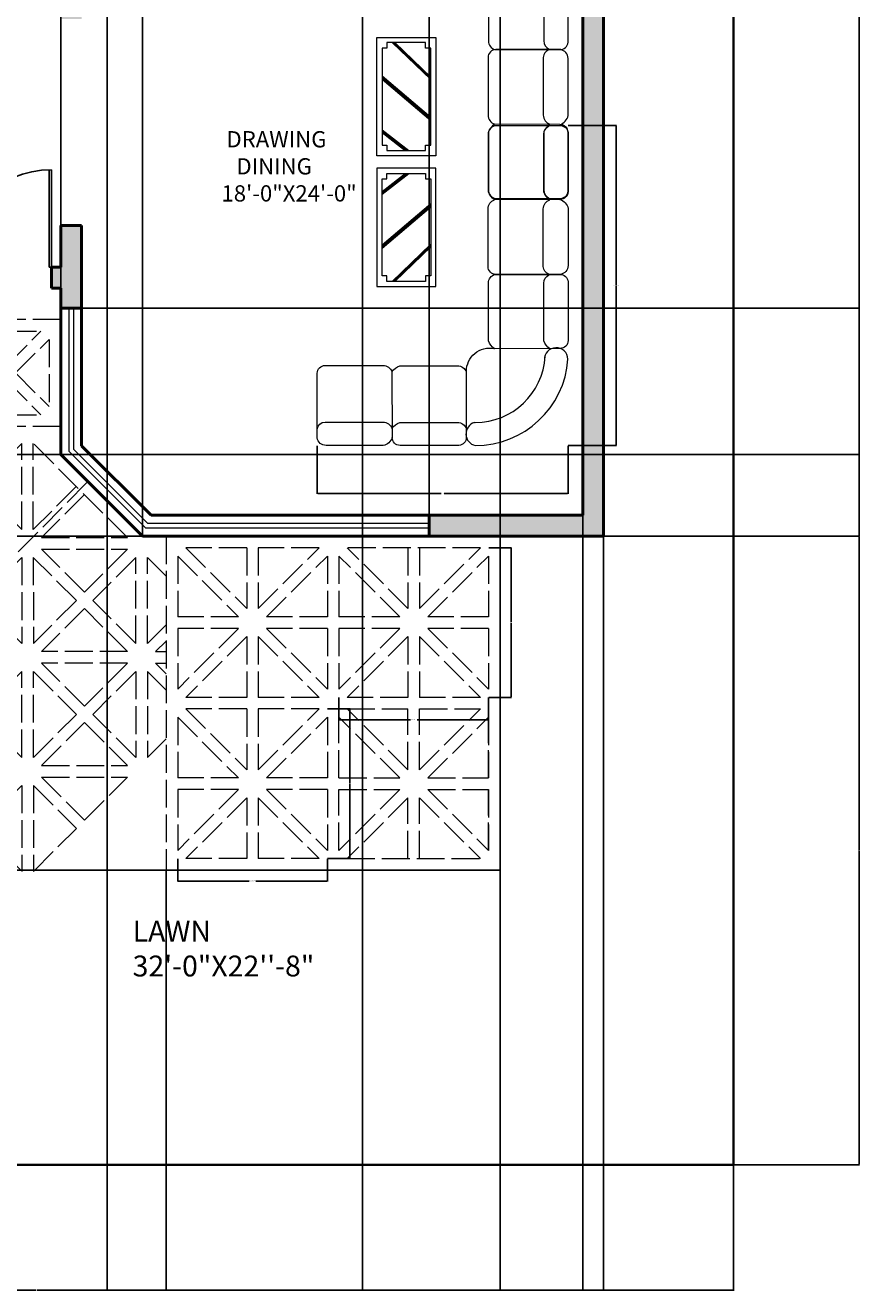
# Model space of a CAD drawing. Units: inches. Extents: x 2447 to 3157, y 2799 to 3988.
# Tile 2 of 9: x 2797 to 3157, y 2799 to 3345. Entities that reach past the tile are written whole.
import ezdxf

# ---------------------------------------------------------------- set-up
doc = ezdxf.new("R2010")
doc.units = ezdxf.units.IN
doc.linetypes.add('ACAD_ISO02W100', pattern=[15, 12, -3])
for name, color, linetype, lineweight in [('A-ANNO-DIMS', 2, 'Continuous', 18), ('A-AREA-IDEN', 7, 'Continuous', 25), ('A-DOOR', 3, 'Continuous', 25), ('A-FLOR-OVHD', 8, 'ACAD_ISO02W100', 18), ('A-FURN', 8, 'Continuous', 18), ('A-GLAZ', 4, 'Continuous', 18), ('A-WALL', 7, 'Continuous', 50), ('A-WALL-PATT', 252, 'Continuous', 13), ('C-PROP', 6, 'Continuous', 35), ('L-PAVE-PATT', 9, 'ACAD_ISO02W100', 13)]:
    doc.layers.add(name, color=color, linetype=linetype, lineweight=lineweight)
doc.styles.get("Standard").update_dxf_attribs({"font": 'arial.ttf'})
doc.dimstyles.get("Standard").update_dxf_attribs({"dimtxt": 0.18, "dimasz": 0.18, "dimexe": 0.18, "dimexo": 0.0625, "dimgap": 0.09, "dimtad": 0, "dimtih": 1, "dimtoh": 1, "dimdec": 4, "dimzin": 0, "dimdsep": 46, "dimtxsty": 'Standard', "dimcen": 0.09, "dimadec": 0, "dimazin": 0, "dimtfac": 1, "dimtdec": 4, "dimtofl": 0, "dimtmove": 0, "dimatfit": 3, "dimfxl": 1, "dimtolj": 1, "dimtzin": 0, "dimarcsym": 0})

# ---------------------------------------------------------------- blocks, each defined once
blk = doc.blocks.new('A$C2F471D6A')
for p, q in [((2696, 2657), (2692, 1940)), ((1797, 841), (2183, 1243)), ((1797, 834), (2190, 1243)), ((1797, 826), (2197, 1243)), ((1797, 819), (2204, 1243)), ((1797, 849), (2175, 1243)), ((2161, 710), (2615, 1243)), ((2169, 710), (2622, 1243)), ((2176, 710), (2630, 1243)), ((2183, 710), (2637, 1243)), ((2190, 710), (2644, 1243)), ((2197, 710), (2651, 1243)), ((2755, 710), (2980, 1001)), ((2763, 710), (2981, 992)), ((2770, 710), (2981, 983)), ((2777, 710), (2981, 973)), ((2784, 710), (2981, 964)), ((807, 818), (90, 821))]:
    blk.add_line(p, q)
for points in [[(0, 1730, -0.393715), (947, 2745)], [(947, 2745, -1), (938, 2487, 1)], [(1061, 1940, 0.132391), (1146, 1873), (1779, 1873, 0.326313), (1875, 1944), (1875, 2657, 0.389129), (1793, 2746), (1150, 2746, 0.426582), (1064, 2657, 0.287811)], [(1061, 2546, 0.132391), (1146, 2479), (1779, 2479, 0.287096), (1869, 2536)], [(1878, 2536, 0.331063), (1960, 2475), (2433, 2475)], [(2433, 2475), (2592, 2475, 0.316456), (2692, 2546, 0.132391), (2777, 2479), (3410, 2479, 0.287096), (3501, 2536)], [(252, 1720), (252, 1729, -0.399385), (979, 2494)], [(813, 1633, 0.469502), (1064, 1935, -1.204519)], [(252, 1720, -0.77294), (0, 1730, -1)], [(257, 559), (257, 718, 0.316456), (187, 818, 0.132391), (254, 903), (254, 1535, 0.326313), (183, 1632), (181, 1632, 0.389129)], [(181, 0, 0.385191), (257, 85), (257, 559)]]:
    blk.add_lwpolyline(points, format="xyb")
blk.add_lwpolyline([(1064, 2657), (1061, 1940)])
for points in [[(2433, 1870), (2592, 1870, 0.316456), (2692, 1940, 0.132391), (2777, 1873), (3410, 1873, 0.326313), (3506, 1944), (3506, 2657, 0.389129), (3425, 2746), (2781, 2746, 0.426582), (2696, 2657, 0.287811), (2596, 2746), (1971, 2746, 0.366167), (1875, 2665), (1875, 1955, 0.414362), (1960, 1870)], [(878, 559), (878, 718, 0.316456), (807, 818, 0.132391), (874, 903), (874, 1535, 0.326313), (804, 1632), (90, 1632, 0.389129), (1, 1550), (1, 906, 0.426582), (90, 821, 0.287811), (1, 721), (1, 96, 0.366167), (83, 0), (792, 0, 0.414362), (878, 85)]]:
    blk.add_lwpolyline(points, format="xyb", close=True)
for points in [[(1742, 652), (1742, 1300), (3038, 1300), (3038, 652)], [(2981, 1186), (2920, 1186), (2920, 1243), (1860, 1243), (1860, 1186), (1797, 1186), (1797, 762), (1860, 762), (1860, 709), (2920, 709), (2920, 762), (2981, 762)]]:
    blk.add_lwpolyline(points, close=True)
blk = doc.blocks.new('DOOR-SWING-42IN')
for p, q in [((0, 0), (0, 42)), ((1, 0), (1, 41.99)), ((1, 0), (0, 0))]:
    blk.add_line(p, q)
blk.add_arc((0, 0), 42, 0, 90)
blk = doc.blocks.new('PAVER-PANEL-RADIAL')
for p, q in [((0, 60.96), (0, 34.75)), ((0, 60.96), (26.22, 34.75)), ((3.54, 64.5), (29.75, 38.29)), ((29.75, 64.5), (3.54, 64.5)), ((29.75, 64.5), (29.75, 38.29)), ((34.75, 64.5), (34.75, 38.29)), ((60.97, 64.5), (34.75, 64.5)), ((34.75, 38.29), (60.97, 64.5)), ((38.29, 34.75), (64.51, 60.96)), ((64.51, 60.96), (64.51, 34.75)), ((26.22, 34.75), (0, 34.75)), ((64.51, 34.75), (38.29, 34.75)), ((0, 29.75), (0, 3.54)), ((26.22, 29.75), (0, 3.54)), ((26.22, 29.75), (0, 29.75)), ((38.29, 29.75), (64.51, 3.54)), ((64.51, 29.75), (38.29, 29.75)), ((64.51, 29.75), (64.51, 3.54)), ((29.75, 26.21), (3.54, 0)), ((29.75, 26.21), (29.75, 0)), ((34.75, 26.21), (34.75, 0)), ((34.75, 26.21), (60.97, 0)), ((29.75, 0), (3.54, 0)), ((60.97, 0), (34.75, 0))]:
    blk.add_line(p, q)
blk = doc.blocks.new('PAVER-PANEL-LINKED')
for p, q in [((0, 60.96), (0, 34.75)), ((26.22, 34.75), (0, 60.96)), ((60.97, 64.5), (3.54, 64.5)), ((29.75, 38.29), (3.54, 64.5)), ((29.75, 64.5), (29.75, 38.29)), ((34.75, 64.5), (34.75, 38.29)), ((34.75, 38.29), (60.97, 64.5)), ((38.29, 34.75), (64.51, 60.96)), ((64.51, 60.96), (64.51, 34.75)), ((26.22, 34.75), (0, 34.75)), ((64.51, 34.75), (38.29, 34.75)), ((0, 29.75), (0, 3.54)), ((26.22, 29.75), (0, 3.54)), ((26.22, 29.75), (0, 29.75)), ((64.51, 29.75), (38.29, 29.75)), ((38.29, 29.75), (64.51, 3.54)), ((64.51, 29.75), (64.51, 3.54)), ((29.75, 26.21), (3.54, 0)), ((29.75, 26.21), (29.75, 0)), ((34.75, 26.21), (34.75, 0)), ((34.75, 26.21), (60.97, 0)), ((29.75, 0), (3.54, 0)), ((60.97, 0), (34.75, 0))]:
    blk.add_line(p, q)
blk = doc.blocks.new('PORCH-PAVER-FOUR-TRIANGLE')
for p, q in [((32.46, 36), (3.54, 36)), ((3.54, 36), (18, 21.54)), ((32.46, 36), (18, 21.54)), ((0, 32.46), (0, 3.54)), ((0, 32.46), (14.46, 18)), ((36, 32.46), (21.54, 18)), ((36, 32.46), (36, 3.54)), ((14.46, 18), (0, 3.54)), ((21.54, 18), (36, 3.54)), ((18, 14.46), (3.54, 0)), ((18, 14.46), (32.46, 0)), ((32.46, 0), (3.54, 0))]:
    blk.add_line(p, q)
blk = doc.blocks.new('*D28')
at = {"layer": 'A-ANNO-DIMS', "color": 0, "lineweight": -2, "transparency": 16777216}
for p, q in [((3031.13, 3301.82), (3051.95, 3301.82)), ((3051.77, 3301.64), (3051.77, 3232.98)), ((3051.77, 3163.96), (3051.77, 3232.62)), ((3031.13, 3163.78), (3051.95, 3163.78))]:
    blk.add_line(p, q, dxfattribs=at)
at = {"layer": 'A-ANNO-DIMS', "color": 0, "transparency": 16777216}
for points in [[(3051.74, 3301.64), (3051.8, 3301.64), (3051.77, 3301.82)], [(3051.74, 3163.96), (3051.8, 3163.96), (3051.77, 3163.78)]]:
    blk.add_solid(points, dxfattribs=at)
at = {"layer": 'Defpoints', "color": 0, "transparency": 16777216}
for p in [(3031.06, 3301.82), (3051.77, 3301.82), (3031.06, 3163.78)]:
    blk.add_point(p, dxfattribs=at)
at = {"layer": 'A-ANNO-DIMS', "color": 0, "transparency": 16777216, "insert": (3051.77, 3232.8), "char_height": 0.18, "attachment_point": 5}
blk.add_mtext('\\A1;SECTIONAL 138 TYP.', dxfattribs=at)
blk = doc.blocks.new('*D29')
at = {"layer": 'A-ANNO-DIMS', "color": 0, "lineweight": -2, "transparency": 16777216}
for p, q in [((2922.95, 3163.72), (2922.95, 3142.9)), ((3031.06, 3163.72), (3031.06, 3142.9)), ((2923.13, 3143.08), (2976.42, 3143.08)), ((3030.88, 3143.08), (2977.6, 3143.08))]:
    blk.add_line(p, q, dxfattribs=at)
at = {"layer": 'A-ANNO-DIMS', "color": 0, "transparency": 16777216}
for points in [[(2923.13, 3143.11), (2923.13, 3143.05), (2922.95, 3143.08)], [(3030.88, 3143.11), (3030.88, 3143.05), (3031.06, 3143.08)]]:
    blk.add_solid(points, dxfattribs=at)
at = {"layer": 'Defpoints', "color": 0, "transparency": 16777216}
for p in [(2922.95, 3163.78), (3031.06, 3163.78), (3031.06, 3143.08)]:
    blk.add_point(p, dxfattribs=at)
at = {"layer": 'A-ANNO-DIMS', "color": 0, "transparency": 16777216, "insert": (2977.01, 3143.08), "char_height": 0.18, "attachment_point": 5}
blk.add_mtext('\\A1;108 TYP.', dxfattribs=at)
blk = doc.blocks.new('*D38')
at = {"layer": 'A-ANNO-DIMS', "color": 0, "lineweight": -2, "transparency": 16777216}
for p, q in [((2932.3, 3055.14), (2932.3, 3045.34)), ((2996.81, 3055.14), (2996.81, 3045.34)), ((2932.48, 3045.52), (2963.08, 3045.52)), ((2996.63, 3045.52), (2966.03, 3045.52))]:
    blk.add_line(p, q, dxfattribs=at)
at = {"layer": 'A-ANNO-DIMS', "color": 0, "transparency": 16777216}
for points in [[(2932.48, 3045.55), (2932.48, 3045.49), (2932.3, 3045.52)], [(2996.63, 3045.55), (2996.63, 3045.49), (2996.81, 3045.52)]]:
    blk.add_solid(points, dxfattribs=at)
at = {"layer": 'Defpoints', "color": 0, "transparency": 16777216}
for p in [(2932.3, 3055.2), (2996.81, 3055.2), (2996.81, 3045.52)]:
    blk.add_point(p, dxfattribs=at)
at = {"layer": 'A-ANNO-DIMS', "color": 0, "transparency": 16777216, "insert": (2964.55, 3045.52), "char_height": 0.18, "attachment_point": 5}
blk.add_mtext('\\A1;LINKED PAVER 65 TYP.', dxfattribs=at)
blk = doc.blocks.new('*D39')
at = {"layer": 'A-ANNO-DIMS', "color": 0, "lineweight": -2, "transparency": 16777216}
for p, q in [((2996.87, 3119.7), (3006.66, 3119.7)), ((3006.48, 3119.52), (3006.48, 3087.63)), ((3006.48, 3055.38), (3006.48, 3087.27)), ((2996.87, 3055.2), (3006.66, 3055.2))]:
    blk.add_line(p, q, dxfattribs=at)
at = {"layer": 'A-ANNO-DIMS', "color": 0, "transparency": 16777216}
for points in [[(3006.45, 3119.52), (3006.51, 3119.52), (3006.48, 3119.7)], [(3006.45, 3055.38), (3006.51, 3055.38), (3006.48, 3055.2)]]:
    blk.add_solid(points, dxfattribs=at)
at = {"layer": 'Defpoints', "color": 0, "transparency": 16777216}
for p in [(2996.81, 3119.7), (3006.48, 3119.7), (2996.81, 3055.2)]:
    blk.add_point(p, dxfattribs=at)
at = {"layer": 'A-ANNO-DIMS', "color": 0, "transparency": 16777216, "insert": (3006.48, 3087.45), "char_height": 0.18, "attachment_point": 5}
blk.add_mtext('\\A1;65 TYP.', dxfattribs=at)
blk = doc.blocks.new('*D40')
at = {"layer": 'A-ANNO-DIMS', "color": 0, "lineweight": -2, "transparency": 16777216}
for p, q in [((2862.79, 2985.64), (2862.79, 2975.84)), ((2927.3, 2985.64), (2927.3, 2975.84)), ((2862.97, 2976.02), (2893.57, 2976.02)), ((2927.12, 2976.02), (2896.52, 2976.02))]:
    blk.add_line(p, q, dxfattribs=at)
at = {"layer": 'A-ANNO-DIMS', "color": 0, "transparency": 16777216}
for points in [[(2862.97, 2976.05), (2862.97, 2975.99), (2862.79, 2976.02)], [(2927.12, 2976.05), (2927.12, 2975.99), (2927.3, 2976.02)]]:
    blk.add_solid(points, dxfattribs=at)
at = {"layer": 'Defpoints', "color": 0, "transparency": 16777216}
for p in [(2862.79, 2985.7), (2927.3, 2985.7), (2927.3, 2976.02)]:
    blk.add_point(p, dxfattribs=at)
at = {"layer": 'A-ANNO-DIMS', "color": 0, "transparency": 16777216, "insert": (2895.04, 2976.02), "char_height": 0.18, "attachment_point": 5}
blk.add_mtext('\\A1;RADIAL PAVER 65 TYP.', dxfattribs=at)
blk = doc.blocks.new('*D41')
at = {"layer": 'A-ANNO-DIMS', "color": 0, "lineweight": -2, "transparency": 16777216}
for p, q in [((2927.36, 3050.2), (2937.15, 3050.2)), ((2936.97, 3050.02), (2936.97, 3018.13)), ((2936.97, 2985.88), (2936.97, 3017.77)), ((2927.36, 2985.7), (2937.15, 2985.7))]:
    blk.add_line(p, q, dxfattribs=at)
at = {"layer": 'A-ANNO-DIMS', "color": 0, "transparency": 16777216}
for points in [[(2936.94, 3050.02), (2937, 3050.02), (2936.97, 3050.2)], [(2936.94, 2985.88), (2937, 2985.88), (2936.97, 2985.7)]]:
    blk.add_solid(points, dxfattribs=at)
at = {"layer": 'Defpoints', "color": 0, "transparency": 16777216}
for p in [(2927.3, 3050.2), (2936.97, 3050.2), (2927.3, 2985.7)]:
    blk.add_point(p, dxfattribs=at)
at = {"layer": 'A-ANNO-DIMS', "color": 0, "transparency": 16777216, "insert": (2936.97, 3017.95), "char_height": 0.18, "attachment_point": 5}
blk.add_mtext('\\A1;65 TYP.', dxfattribs=at)
blk = doc.blocks.new('*D44')
at = {"layer": 'A-ANNO-DIMS', "color": 0, "lineweight": -2, "transparency": 16777216}
for p, q in [((2501.37, 2853.64), (2501.37, 2799.37)), ((3102.37, 2853.64), (3102.37, 2799.37)), ((2501.55, 2799.55), (2801.6, 2799.55)), ((3102.19, 2799.55), (2802.14, 2799.55))]:
    blk.add_line(p, q, dxfattribs=at)
at = {"layer": 'A-ANNO-DIMS', "color": 0, "transparency": 16777216}
for points in [[(2501.55, 2799.58), (2501.55, 2799.52), (2501.37, 2799.55)], [(3102.19, 2799.58), (3102.19, 2799.52), (3102.37, 2799.55)]]:
    blk.add_solid(points, dxfattribs=at)
at = {"layer": 'Defpoints', "color": 0, "transparency": 16777216}
for p in [(2501.37, 2853.7), (3102.37, 2853.7), (3102.37, 2799.55)]:
    blk.add_point(p, dxfattribs=at)
at = {"layer": 'A-ANNO-DIMS', "color": 0, "transparency": 16777216, "insert": (2801.87, 2799.55), "char_height": 0.18, "attachment_point": 5}
blk.add_mtext('\\A1;601', dxfattribs=at)
blk = doc.blocks.new('*D47')
at = {"layer": 'A-ANNO-DIMS', "color": 0, "lineweight": -2, "transparency": 16777216}
for p, q in [((2798.43, 3849.7), (3156.7, 3849.7)), ((3156.52, 3849.52), (3156.52, 3487.38)), ((3156.52, 3124.88), (3156.52, 3487.02)), ((3046.43, 3124.7), (3156.7, 3124.7))]:
    blk.add_line(p, q, dxfattribs=at)
at = {"layer": 'A-ANNO-DIMS', "color": 0, "transparency": 16777216}
for points in [[(3156.49, 3849.52), (3156.55, 3849.52), (3156.52, 3849.7)], [(3156.49, 3124.88), (3156.55, 3124.88), (3156.52, 3124.7)]]:
    blk.add_solid(points, dxfattribs=at)
at = {"layer": 'Defpoints', "color": 0, "transparency": 16777216}
for p in [(2798.37, 3849.7), (3156.52, 3849.7), (3046.37, 3124.7)]:
    blk.add_point(p, dxfattribs=at)
at = {"layer": 'A-ANNO-DIMS', "color": 0, "transparency": 16777216, "insert": (3156.52, 3487.2), "char_height": 0.18, "attachment_point": 5}
blk.add_mtext('\\A1;725', dxfattribs=at)
blk = doc.blocks.new('*D48')
at = {"layer": 'A-ANNO-DIMS', "color": 0, "lineweight": -2, "transparency": 16777216}
for p, q in [((3046.43, 3124.7), (3156.7, 3124.7)), ((3156.52, 3124.52), (3156.52, 2989.38)), ((3156.52, 2853.88), (3156.52, 2989.02)), ((3102.43, 2853.7), (3156.7, 2853.7))]:
    blk.add_line(p, q, dxfattribs=at)
at = {"layer": 'A-ANNO-DIMS', "color": 0, "transparency": 16777216}
for points in [[(3156.49, 3124.52), (3156.55, 3124.52), (3156.52, 3124.7)], [(3156.49, 2853.88), (3156.55, 2853.88), (3156.52, 2853.7)]]:
    blk.add_solid(points, dxfattribs=at)
at = {"layer": 'Defpoints', "color": 0, "transparency": 16777216}
for p in [(3046.37, 3124.7), (3102.37, 2853.7), (3156.52, 2853.7)]:
    blk.add_point(p, dxfattribs=at)
at = {"layer": 'A-ANNO-DIMS', "color": 0, "transparency": 16777216, "insert": (3156.52, 2989.2), "char_height": 0.18, "attachment_point": 5}
blk.add_mtext('\\A1;271', dxfattribs=at)
blk = doc.blocks.new('*D50')
at = {"layer": 'A-ANNO-DIMS', "color": 0, "lineweight": -2, "transparency": 16777216}
for p, q in [((2832.46, 3897.64), (2832.46, 2799.37)), ((2942.46, 3897.64), (2942.46, 2799.37)), ((2832.64, 2799.55), (2887.18, 2799.55)), ((2942.28, 2799.55), (2887.74, 2799.55))]:
    blk.add_line(p, q, dxfattribs=at)
at = {"layer": 'A-ANNO-DIMS', "color": 0, "transparency": 16777216}
for points in [[(2832.64, 2799.58), (2832.64, 2799.52), (2832.46, 2799.55)], [(2942.28, 2799.58), (2942.28, 2799.52), (2942.46, 2799.55)]]:
    blk.add_solid(points, dxfattribs=at)
at = {"layer": 'Defpoints', "color": 0, "transparency": 16777216}
for p in [(2832.46, 3897.7), (2942.46, 3897.7), (2942.46, 2799.55)]:
    blk.add_point(p, dxfattribs=at)
at = {"layer": 'A-ANNO-DIMS', "color": 0, "transparency": 16777216, "insert": (2887.46, 2799.55), "char_height": 0.18, "attachment_point": 5}
blk.add_mtext('\\A1;110', dxfattribs=at)
blk = doc.blocks.new('*D53')
at = {"layer": 'A-ANNO-DIMS', "color": 0, "lineweight": -2, "transparency": 16777216}
for p, q in [((3037.37, 3133.64), (3037.37, 2799.37)), ((3046.37, 3124.64), (3046.37, 2799.37)), ((3037.55, 2799.55), (3041.72, 2799.55)), ((3046.19, 2799.55), (3042.02, 2799.55))]:
    blk.add_line(p, q, dxfattribs=at)
at = {"layer": 'A-ANNO-DIMS', "color": 0, "transparency": 16777216}
for points in [[(3037.55, 2799.58), (3037.55, 2799.52), (3037.37, 2799.55)], [(3046.19, 2799.58), (3046.19, 2799.52), (3046.37, 2799.55)]]:
    blk.add_solid(points, dxfattribs=at)
at = {"layer": 'Defpoints', "color": 0, "transparency": 16777216}
for p in [(3037.37, 3133.7), (3046.37, 3124.7), (3046.37, 2799.55)]:
    blk.add_point(p, dxfattribs=at)
at = {"layer": 'A-ANNO-DIMS', "color": 0, "transparency": 16777216, "insert": (3041.87, 2799.55), "char_height": 0.18, "attachment_point": 5}
blk.add_mtext('\\A1;9', dxfattribs=at)
blk = doc.blocks.new('*D70')
at = {"layer": 'A-ANNO-DIMS', "color": 0, "lineweight": -2, "transparency": 16777216}
for p, q in [((3001.81, 2980.76), (3001.81, 3988.03)), ((3001.99, 3987.85), (3051.63, 3987.85)), ((3102.19, 3987.85), (3052.54, 3987.85)), ((3102.37, 2853.76), (3102.37, 3988.03))]:
    blk.add_line(p, q, dxfattribs=at)
at = {"layer": 'A-ANNO-DIMS', "color": 0, "transparency": 16777216}
for points in [[(3001.99, 3987.88), (3001.99, 3987.82), (3001.81, 3987.85)], [(3102.19, 3987.88), (3102.19, 3987.82), (3102.37, 3987.85)]]:
    blk.add_solid(points, dxfattribs=at)
at = {"layer": 'Defpoints', "color": 0, "transparency": 16777216}
for p in [(3102.37, 3987.85), (3001.81, 2980.7), (3102.37, 2853.7)]:
    blk.add_point(p, dxfattribs=at)
at = {"layer": 'A-ANNO-DIMS', "color": 0, "transparency": 16777216, "insert": (3052.09, 3987.85), "char_height": 0.18, "attachment_point": 5}
blk.add_mtext('\\A1;100.56', dxfattribs=at)
blk = doc.blocks.new('*D71')
at = {"layer": 'A-ANNO-DIMS', "color": 0, "lineweight": -2, "transparency": 16777216}
for p, q in [((3001.74, 2980.7), (2447.04, 2980.7)), ((2447.22, 2980.52), (2447.22, 2917.38)), ((2447.22, 2853.88), (2447.22, 2917.02)), ((3102.3, 2853.7), (2447.04, 2853.7))]:
    blk.add_line(p, q, dxfattribs=at)
at = {"layer": 'A-ANNO-DIMS', "color": 0, "transparency": 16777216}
for points in [[(2447.19, 2980.52), (2447.25, 2980.52), (2447.22, 2980.7)], [(2447.19, 2853.88), (2447.25, 2853.88), (2447.22, 2853.7)]]:
    blk.add_solid(points, dxfattribs=at)
at = {"layer": 'Defpoints', "color": 0, "transparency": 16777216}
for p in [(3001.81, 2980.7), (2447.22, 2853.7), (3102.37, 2853.7)]:
    blk.add_point(p, dxfattribs=at)
at = {"layer": 'A-ANNO-DIMS', "color": 0, "transparency": 16777216, "insert": (2447.22, 2917.2), "char_height": 0.18, "attachment_point": 5}
blk.add_mtext('\\A1;127', dxfattribs=at)
blk = doc.blocks.new('*D72')
at = {"layer": 'A-ANNO-DIMS', "color": 0, "lineweight": -2, "transparency": 16777216}
for p, q in [((2857.79, 2980.64), (2857.79, 2799.37)), ((3001.81, 2980.64), (3001.81, 2799.37)), ((2857.97, 2799.55), (2929.34, 2799.55)), ((3001.63, 2799.55), (2930.25, 2799.55))]:
    blk.add_line(p, q, dxfattribs=at)
at = {"layer": 'A-ANNO-DIMS', "color": 0, "transparency": 16777216}
for points in [[(2857.97, 2799.58), (2857.97, 2799.52), (2857.79, 2799.55)], [(3001.63, 2799.58), (3001.63, 2799.52), (3001.81, 2799.55)]]:
    blk.add_solid(points, dxfattribs=at)
at = {"layer": 'Defpoints', "color": 0, "transparency": 16777216}
for p in [(2857.79, 2980.7), (3001.81, 2980.7), (3001.81, 2799.55)]:
    blk.add_point(p, dxfattribs=at)
at = {"layer": 'A-ANNO-DIMS', "color": 0, "transparency": 16777216, "insert": (2929.8, 2799.55), "char_height": 0.18, "attachment_point": 5}
blk.add_mtext('\\A1;144.02', dxfattribs=at)
blk = doc.blocks.new('*D73')
at = {"layer": 'A-ANNO-DIMS', "color": 0, "lineweight": -2, "transparency": 16777216}
for p, q in [((2812.37, 3160.03), (2812.37, 3988.03)), ((2812.55, 3987.85), (2829.61, 3987.85)), ((2847.46, 3987.85), (2830.4, 3987.85)), ((2847.64, 3124.76), (2847.64, 3988.03))]:
    blk.add_line(p, q, dxfattribs=at)
at = {"layer": 'A-ANNO-DIMS', "color": 0, "transparency": 16777216}
for points in [[(2812.55, 3987.88), (2812.55, 3987.82), (2812.37, 3987.85)], [(2847.46, 3987.88), (2847.46, 3987.82), (2847.64, 3987.85)]]:
    blk.add_solid(points, dxfattribs=at)
at = {"layer": 'Defpoints', "color": 0, "transparency": 16777216}
for p in [(2847.64, 3987.85), (2812.37, 3159.97), (2847.64, 3124.7)]:
    blk.add_point(p, dxfattribs=at)
at = {"layer": 'A-ANNO-DIMS', "color": 0, "transparency": 16777216, "insert": (2830, 3987.85), "char_height": 0.18, "attachment_point": 5}
blk.add_mtext('\\A1;35.27', dxfattribs=at)
blk = doc.blocks.new('*D74')
at = {"layer": 'A-ANNO-DIMS', "color": 0, "lineweight": -2, "transparency": 16777216}
for p, q in [((2812.3, 3159.97), (2447.04, 3159.97)), ((2447.22, 3159.79), (2447.22, 3142.52)), ((2447.22, 3124.88), (2447.22, 3142.15)), ((2847.58, 3124.7), (2447.04, 3124.7))]:
    blk.add_line(p, q, dxfattribs=at)
at = {"layer": 'A-ANNO-DIMS', "color": 0, "transparency": 16777216}
for points in [[(2447.19, 3159.79), (2447.25, 3159.79), (2447.22, 3159.97)], [(2447.19, 3124.88), (2447.25, 3124.88), (2447.22, 3124.7)]]:
    blk.add_solid(points, dxfattribs=at)
at = {"layer": 'Defpoints', "color": 0, "transparency": 16777216}
for p in [(2812.37, 3159.97), (2447.22, 3124.7), (2847.64, 3124.7)]:
    blk.add_point(p, dxfattribs=at)
at = {"layer": 'A-ANNO-DIMS', "color": 0, "transparency": 16777216, "insert": (2447.22, 3142.34), "char_height": 0.18, "attachment_point": 5}
blk.add_mtext('\\A1;35.27', dxfattribs=at)
blk = doc.blocks.new('*D75')
at = {"layer": 'A-ANNO-DIMS', "color": 0, "lineweight": -2, "transparency": 16777216}
for p, q in [((2812.43, 3223.07), (3156.7, 3223.07)), ((3156.52, 3222.89), (3156.52, 3191.7)), ((3156.52, 3160.15), (3156.52, 3191.34)), ((2812.43, 3159.97), (3156.7, 3159.97))]:
    blk.add_line(p, q, dxfattribs=at)
at = {"layer": 'A-ANNO-DIMS', "color": 0, "transparency": 16777216}
for points in [[(3156.49, 3222.89), (3156.55, 3222.89), (3156.52, 3223.07)], [(3156.49, 3160.15), (3156.55, 3160.15), (3156.52, 3159.97)]]:
    blk.add_solid(points, dxfattribs=at)
at = {"layer": 'Defpoints', "color": 0, "transparency": 16777216}
for p in [(2812.37, 3223.07), (3156.52, 3223.07), (2812.37, 3159.97)]:
    blk.add_point(p, dxfattribs=at)
at = {"layer": 'A-ANNO-DIMS', "color": 0, "transparency": 16777216, "insert": (3156.52, 3191.52), "char_height": 0.18, "attachment_point": 5}
blk.add_mtext('\\A1;63.1', dxfattribs=at)
blk = doc.blocks.new('*D76')
at = {"layer": 'A-ANNO-DIMS', "color": 0, "lineweight": -2, "transparency": 16777216}
for p, q in [((2847.64, 3124.76), (2847.64, 3988.03)), ((2847.82, 3987.85), (2908.95, 3987.85)), ((2970.99, 3987.85), (2909.86, 3987.85)), ((2971.17, 3124.76), (2971.17, 3988.03))]:
    blk.add_line(p, q, dxfattribs=at)
at = {"layer": 'A-ANNO-DIMS', "color": 0, "transparency": 16777216}
for points in [[(2847.82, 3987.88), (2847.82, 3987.82), (2847.64, 3987.85)], [(2970.99, 3987.88), (2970.99, 3987.82), (2971.17, 3987.85)]]:
    blk.add_solid(points, dxfattribs=at)
at = {"layer": 'Defpoints', "color": 0, "transparency": 16777216}
for p in [(2971.17, 3987.85), (2847.64, 3124.7), (2971.17, 3124.7)]:
    blk.add_point(p, dxfattribs=at)
at = {"layer": 'A-ANNO-DIMS', "color": 0, "transparency": 16777216, "insert": (2909.4, 3987.85), "char_height": 0.18, "attachment_point": 5}
blk.add_mtext('\\A1;123.53', dxfattribs=at)

msp = doc.modelspace()

# ---------------------------------------------------------------- hatches: boundary and pattern name
at = {"layer": 'A-WALL-PATT'}
h = msp.add_hatch(color=256, dxfattribs=at)
h.dxf.hatch_style = 1
h.paths.add_polyline_path([(2570.3672, 3550.7002), (2726.3672, 3550.7002), (2726.3672, 3370.7002), (2722.3672, 3370.7002), (2722.3672, 3365.7002), (2739.3672, 3365.7002), (2739.3672, 3374.7002), (2735.3672, 3374.7002), (2735.3672, 3563.7002), (2726.3672, 3563.7002), (2726.3672, 3559.7002), (2570.3672, 3559.7002), (2570.3672, 3599.2479), (2561.3672, 3599.2479), (2561.3672, 3508.7002), (2570.3672, 3508.7002)])
h.paths.add_polyline_path([(2570.3672, 3412.7002), (2561.3672, 3412.7002), (2561.3672, 3331.9279), (2570.3672, 3331.9279), (2570.3672, 3365.7002), (2666.3672, 3365.7002), (2666.3672, 3361.7002), (2671.3672, 3361.7002), (2671.3672, 3365.7002), (2686.3672, 3365.7002), (2686.3672, 3370.7002), (2570.3672, 3370.7002)])
h.paths.add_polyline_path([(2965.3672, 3430.7002), (2961.3672, 3430.7002), (2961.3672, 3434.7002), (2952.3672, 3434.7002), (2952.3672, 3430.7002), (2847.6393, 3430.7002), (2812.3672, 3395.4282), (2812.3672, 3374.7002), (2781.3672, 3374.7002), (2781.3672, 3365.7002), (2812.3672, 3365.7002), (2812.3672, 3347.7002), (2821.3672, 3347.7002), (2821.3672, 3391.7002), (2851.3672, 3421.7002), (2965.3672, 3421.7002)])
h.paths.add_polyline_path([(3046.3672, 3430.7002), (3033.3672, 3430.7002), (3033.3672, 3421.7002), (3037.3672, 3421.7002), (3037.3672, 3133.7002), (2971.1661, 3133.7002), (2971.1661, 3124.7002), (3046.3672, 3124.7002)])
h.paths.add_polyline_path([(3046.3672, 3825.7002), (3005.5801, 3825.7002), (3005.5801, 3816.7002), (3037.3672, 3816.7002), (3037.3672, 3655.7002), (2940.3672, 3655.7002), (2940.3672, 3646.7002), (3037.3672, 3646.7002), (3037.3672, 3514.7002), (3033.3672, 3514.7002), (3033.3672, 3505.7002), (3046.3672, 3505.7002)])
h.paths.add_polyline_path([(2821.3672, 3258.7002), (2812.3672, 3258.7002), (2812.3672, 3240.7002), (2808.3672, 3240.7002), (2808.3672, 3231.7002), (2812.3672, 3231.7002), (2812.3672, 3223.0688), (2821.3672, 3223.0688)])
h.paths.add_polyline_path([(2766.3672, 3240.7002), (2707.3672, 3240.7002), (2707.3672, 3234.4466, -1), (2570.3672, 3234.4466), (2570.3672, 3240.5271), (2561.3672, 3240.5271), (2561.3672, 3234.4466, 0.98243292), (2716.3185, 3231.7002), (2766.3672, 3231.7002)])
h.paths.add_polyline_path([(2570.3672, 3307.9279), (2561.3672, 3307.9279), (2561.3672, 3281.7773), (2570.3672, 3281.7773), (2570.3672, 3284.7002), (2671.3672, 3284.7002), (2671.3672, 3331.7002), (2666.3672, 3331.7002), (2666.3672, 3293.7002), (2570.3672, 3293.7002)])
h.paths.add_polyline_path([(2570.3672, 3739.7002), (2574.3672, 3739.7002), (2574.3672, 3744.7002), (2570.3672, 3744.7002), (2570.3672, 3840.7002), (2614.3672, 3840.7002), (2614.3672, 3849.7002), (2561.3672, 3849.7002), (2561.3672, 3671.2479), (2570.3672, 3671.2479)])
h.paths.add_polyline_path([(2735.3672, 3840.7002), (2789.3672, 3840.7002), (2789.3672, 3816.7002), (2798.3672, 3816.7002), (2798.3672, 3849.7002), (2679.3672, 3849.7002), (2679.3672, 3840.7002), (2726.3672, 3840.7002), (2726.3672, 3778.7002), (2735.3672, 3778.7002)])
h.paths.add_polyline_path([(2651.3672, 3840.7002), (2655.3672, 3840.7002), (2655.3672, 3849.7002), (2638.3672, 3849.7002), (2638.3672, 3840.7002), (2642.3672, 3840.7002), (2642.3672, 3744.7002), (2610.3672, 3744.7002), (2610.3672, 3739.7002), (2726.3672, 3739.7002), (2726.3672, 3599.7002), (2735.3672, 3599.7002), (2735.3672, 3622.7002), (2739.3672, 3622.7002), (2739.3672, 3631.7002), (2735.3672, 3631.7002), (2735.3672, 3748.7002), (2726.3672, 3748.7002), (2726.3672, 3744.7002), (2651.3672, 3744.7002)])
h.paths.add_polyline_path([(2900.3672, 3816.7002), (2904.3672, 3816.7002), (2904.3672, 3825.7002), (2882.3672, 3825.7002), (2882.3672, 3816.7002), (2891.3672, 3816.7002), (2891.3672, 3650.4282), (2872.6393, 3631.7002), (2775.3672, 3631.7002), (2775.3672, 3622.7002), (2876.3672, 3622.7002), (2900.3672, 3646.7002), (2904.3672, 3646.7002), (2904.3672, 3655.7002), (2900.3672, 3655.7002)])
h.paths.add_polyline_path([(2957.5801, 3825.7002), (2940.3672, 3825.7002), (2940.3672, 3816.7002), (2957.5801, 3816.7002)], flags=17)

# ---------------------------------------------------------------- linework, layer by layer
at = {"layer": 'A-FLOR-OVHD'}
msp.add_line((2823.6143, 3147.799), (2725.011, 3048.248), dxfattribs=at)
at = {"layer": 'A-GLAZ'}
for p, q in [((2815.8672, 3223.0688), (2815.8672, 3161.4221)), ((2817.8672, 3223.0688), (2817.8672, 3162.2505)), ((2815.8672, 3161.4221), (2849.0891, 3128.2002)), ((2817.8672, 3162.2505), (2849.9175, 3130.2002)), ((2971.1661, 3128.2002), (2849.0891, 3128.2002)), ((2971.1661, 3130.2002), (2849.9175, 3130.2002))]:
    msp.add_line(p, q, dxfattribs=at)
at = {"layer": 'A-WALL'}
for p, q in [((3046.3672, 3825.7002), (3046.3672, 3124.7002)), ((3037.3672, 3421.7002), (3037.3672, 3133.7002)), ((2812.3672, 3258.7002), (2821.3672, 3258.7002)), ((2812.3672, 3258.7002), (2812.3672, 3240.7002)), ((2821.3672, 3258.7002), (2821.3672, 3163.7002)), ((2808.3672, 3240.7002), (2808.3672, 3231.7002)), ((2808.3672, 3240.7002), (2812.3672, 3240.7002)), ((2808.3672, 3231.7002), (2812.3672, 3231.7002)), ((2812.3672, 3231.7002), (2812.3672, 3159.9723)), ((2812.3672, 3223.0688), (2821.3672, 3223.0688)), ((2812.3672, 3159.9723), (2847.6393, 3124.7002)), ((2821.3672, 3163.7002), (2851.3672, 3133.7002)), ((3037.3672, 3133.7002), (2851.3672, 3133.7002)), ((2971.1661, 3133.7002), (2971.1661, 3124.7002)), ((3046.3672, 3124.7002), (2847.6393, 3124.7002))]:
    msp.add_line(p, q, dxfattribs=at)
at = {"layer": 'C-PROP'}
for p in [(3102.3672, 3933.7002), (2501.3672, 2853.7002)]:
    msp.add_line(p, (3102.3672, 2853.7002), dxfattribs=at)
at = {"layer": 'L-PAVE-PATT'}
for p, q in [((2812.3672, 3218.0737), (2714.618, 3218.0737)), ((2812.3672, 3172.0737), (2684.8659, 3172.0737)), ((2857.7901, 3124.7002), (2857.7901, 2980.7002)), ((3001.807, 3124.7002), (3001.807, 2980.7002)), ((2844.7159, 3115.553), (2826.1793, 3097.0164)), ((2844.7185, 3078.4771), (2844.7159, 3115.553)), ((2849.7185, 3078.4768), (2849.7159, 3115.5526)), ((2857.7901, 3107.4784), (2849.7159, 3115.5526)), ((2844.7185, 3078.4771), (2826.1793, 3097.0164)), ((2822.6437, 3093.4808), (2804.1071, 3074.9442)), ((2841.183, 3074.9416), (2822.6437, 3093.4808)), ((2857.7901, 3086.5484), (2849.7185, 3078.4768)), ((2857.7901, 3079.4773), (2853.254, 3074.9412)), ((2841.183, 3074.9416), (2804.1071, 3074.9442)), ((2853.254, 3074.9412), (2857.7901, 3074.9409)), ((2822.6467, 3051.405), (2804.1075, 3069.9442)), ((2841.1833, 3069.9416), (2804.1075, 3069.9442)), ((2841.1833, 3069.9416), (2822.6467, 3051.405)), ((2853.2544, 3069.9412), (2857.7901, 3069.9409)), ((2857.7901, 3065.4055), (2853.2544, 3069.9412)), ((2844.7188, 3066.4061), (2826.1822, 3047.8695)), ((2844.7188, 3066.4061), (2844.7215, 3029.3302)), ((2857.7901, 3058.3345), (2849.7188, 3066.4057)), ((2849.7188, 3066.4057), (2849.7215, 3029.3299)), ((2844.7215, 3029.3302), (2826.1822, 3047.8695)), ((2996.807, 3046.665), (2996.807, 3020.4502)), ((2857.7901, 3037.3985), (2849.7215, 3029.3299)), ((2996.807, 3015.4502), (2996.807, 2989.2355)), ((3001.807, 2980.7002), (2857.7901, 2980.7002))]:
    msp.add_line(p, q, dxfattribs=at)

# ---------------------------------------------------------------- block references
at = {"layer": 'A-DOOR', "extrusion": (0, 0, -1), "zscale": -1}
msp.add_blockref('DOOR-SWING-42IN', (-2808.3672, 3240.7002), dxfattribs=at)
at = {"layer": 'A-FURN', "yscale": 0.0393700787401575, "zscale": 0.0393700787401575, "rotation": 270}
for p, xscale in [((2922.9523, 3408.3287), 0.0393700787401575), ((2922.9523, 3163.7823), -0.0393700787401575)]:
    msp.add_blockref('A$C2F471D6A', p, dxfattribs=dict(at, xscale=xscale))
at = {"layer": 'L-PAVE-PATT'}
for name, p, rotation in [('PORCH-PAVER-FOUR-TRIANGLE', (2807.367, 3177.0735), 89.99999999999523), ('PAVER-PANEL-LINKED', (2752.4576, 3121.5938), 315.0000000000008), ('PAVER-PANEL-LINKED', (2843.686, 3023.295), 134.9999999999991), ('PAVER-PANEL-LINKED', (2996.8065, 3050.2005), 180)]:
    msp.add_blockref(name, p, dxfattribs=dict(at, rotation=rotation))
for name, p in [('PAVER-PANEL-RADIAL', (2862.79, 3055.2)), ('PAVER-PANEL-LINKED', (2932.299, 3055.2)), ('PAVER-PANEL-RADIAL', (2862.79, 2985.7))]:
    msp.add_blockref(name, p, dxfattribs=at)

# ---------------------------------------------------------------- texts
at = {"layer": 'A-AREA-IDEN', "attachment_point": 1}
for s, width, insert, char_height in [(' DRAWING\\P   DINING\\P18\'-0"X24\'-0"', 93.099677, (2881.6747, 3299.3597), 7), ('LAWN\\P32\'-0"X22\'\'-8"', 92.130589, (2843.3703, 2958.8685), 9)]:
    msp.add_mtext_dynamic_manual_height_columns(s, width=width, gutter_width=12.5, heights=[0], dxfattribs=dict(at, insert=insert, char_height=char_height))

# ---------------------------------------------------------------- dimensions: what is measured, and where the dimension line sits
at = {"layer": 'A-ANNO-DIMS'}
for base, p1, p2, override, picture, middle in [((2847.6393, 3987.8502), (2812.3672, 3159.9723), (2847.6393, 3124.7002), {"dimdec": 2, "dimlfac": 1, "dimrnd": 0, "dimzin": 0, "dimdsep": 46, "dimlunit": 2}, '*D73', (2830.0033, 3987.8502)), ((2971.1661, 3987.8502), (2847.6393, 3124.7002), (2971.1661, 3124.7002), {"dimdec": 2, "dimlfac": 1, "dimrnd": 0, "dimzin": 0, "dimdsep": 46, "dimlunit": 2}, '*D76', (2909.4027, 3987.8502)), ((3102.3672, 3987.8502), (3001.807, 2980.7002), (3102.3672, 2853.7002), {"dimdec": 2, "dimlfac": 1, "dimrnd": 0, "dimzin": 0, "dimdsep": 46, "dimlunit": 2}, '*D70', (3052.0871, 3987.8502)), ((2942.456, 2799.5502), (2832.456, 3897.7002), (2942.456, 3897.7002), {"dimdec": 0, "dimlfac": 1, "dimrnd": 0, "dimzin": 0, "dimdsep": 46, "dimlunit": 2}, '*D50', (2887.456, 2799.5502)), ((3046.3672, 2799.5502), (3037.3672, 3133.7002), (3046.3672, 3124.7002), {"dimdec": 0, "dimlfac": 1, "dimrnd": 0, "dimzin": 0, "dimdsep": 46, "dimlunit": 2}, '*D53', (3041.8672, 2799.5502)), ((3001.807, 2799.5502), (2857.7901, 2980.7002), (3001.807, 2980.7002), {"dimdec": 2, "dimlfac": 1, "dimrnd": 0, "dimzin": 0, "dimdsep": 46, "dimlunit": 2}, '*D72', (2929.7985, 2799.5502)), ((3102.3672, 2799.5502), (2501.3672, 2853.7002), (3102.3672, 2853.7002), {"dimdec": 0, "dimlfac": 1, "dimrnd": 0, "dimzin": 0, "dimdsep": 46, "dimlunit": 2}, '*D44', (2801.8672, 2799.5502))]:
    dim = msp.add_linear_dim(base=base, p1=p1, p2=p2, dimstyle='Standard', override=override, dxfattribs=at)
    dim.commit()
    dim.dimension.update_dxf_attribs({"geometry": picture, "text_midpoint": middle})
for base, p1, p2, override, picture, middle in [((3156.5172, 3849.7002), (3046.3672, 3124.7002), (2798.3672, 3849.7002), {"dimdec": 0, "dimlfac": 1, "dimrnd": 0, "dimzin": 0, "dimdsep": 46, "dimlunit": 2}, '*D47', (3156.5172, 3487.2002)), ((3156.5172, 3223.0688), (2812.3672, 3159.9723), (2812.3672, 3223.0688), {"dimdec": 1, "dimlfac": 1, "dimrnd": 0, "dimzin": 0, "dimdsep": 46, "dimlunit": 2}, '*D75', (3156.5172, 3191.5205)), ((2447.2172, 3124.7002), (2812.3672, 3159.9723), (2847.6393, 3124.7002), {"dimdec": 2, "dimlfac": 1, "dimrnd": 0, "dimzin": 0, "dimdsep": 46, "dimlunit": 2}, '*D74', (2447.2172, 3142.3363)), ((3156.5172, 2853.7002), (3046.3672, 3124.7002), (3102.3672, 2853.7002), {"dimdec": 0, "dimlfac": 1, "dimrnd": 0, "dimzin": 0, "dimdsep": 46, "dimlunit": 2}, '*D48', (3156.5172, 2989.2002)), ((2447.2172, 2853.7002), (3001.807, 2980.7002), (3102.3672, 2853.7002), {"dimdec": 0, "dimlfac": 1, "dimrnd": 0, "dimzin": 0, "dimdsep": 46, "dimlunit": 2}, '*D71', (2447.2172, 2917.2002))]:
    dim = msp.add_linear_dim(base=base, p1=p1, p2=p2, angle=90, dimstyle='Standard', override=override, dxfattribs=at)
    dim.commit()
    dim.dimension.update_dxf_attribs({"geometry": picture, "text_midpoint": middle})
for base, p1, p2, text, picture, middle in [((3051.769, 3301.8164), (3031.0639, 3163.7823), (3031.0639, 3301.8164), 'SECTIONAL <> TYP.', '*D28', (3051.769, 3232.7993)), ((3006.483232639, 3119.7002418708), (2996.8069665467, 3055.2002418708), (2996.8069665467, 3119.7002418708), '<> TYP.', '*D39', (3006.483232639, 3087.4502418708)), ((2936.9747920238, 3050.2002418708), (2927.2985259315, 2985.7002418708), (2927.2985259315, 3050.2002418708), '<> TYP.', '*D41', (2936.9747920238, 3017.9502418708))]:
    dim = msp.add_linear_dim(base=base, p1=p1, p2=p2, angle=90, text=text, dimstyle='Standard', override={"dimdec": 0, "dimlfac": 1, "dimrnd": 0, "dimzin": 0, "dimdsep": 46, "dimlunit": 2}, dxfattribs=at)
    dim.commit()
    dim.dimension.update_dxf_attribs({"geometry": picture, "text_midpoint": middle})
for base, p1, p2, text, picture, middle in [((3031.0639, 3143.0772), (2922.9523, 3163.7823), (3031.0639, 3163.7823), '<> TYP.', '*D29', (2977.0081, 3143.0772)), ((2996.807, 3045.524), (2932.2985, 3055.2002), (2996.807, 3055.2002), 'LINKED PAVER <> TYP.', '*D38', (2964.5527, 3045.524)), ((2927.2985, 2976.024), (2862.7901, 2985.7002), (2927.2985, 2985.7002), 'RADIAL PAVER <> TYP.', '*D40', (2895.0443, 2976.024))]:
    dim = msp.add_linear_dim(base=base, p1=p1, p2=p2, text=text, dimstyle='Standard', override={"dimdec": 0, "dimlfac": 1, "dimrnd": 0, "dimzin": 0, "dimdsep": 46, "dimlunit": 2}, dxfattribs=at)
    dim.commit()
    dim.dimension.update_dxf_attribs({"geometry": picture, "text_midpoint": middle})

doc.saveas('drawing.dxf')
